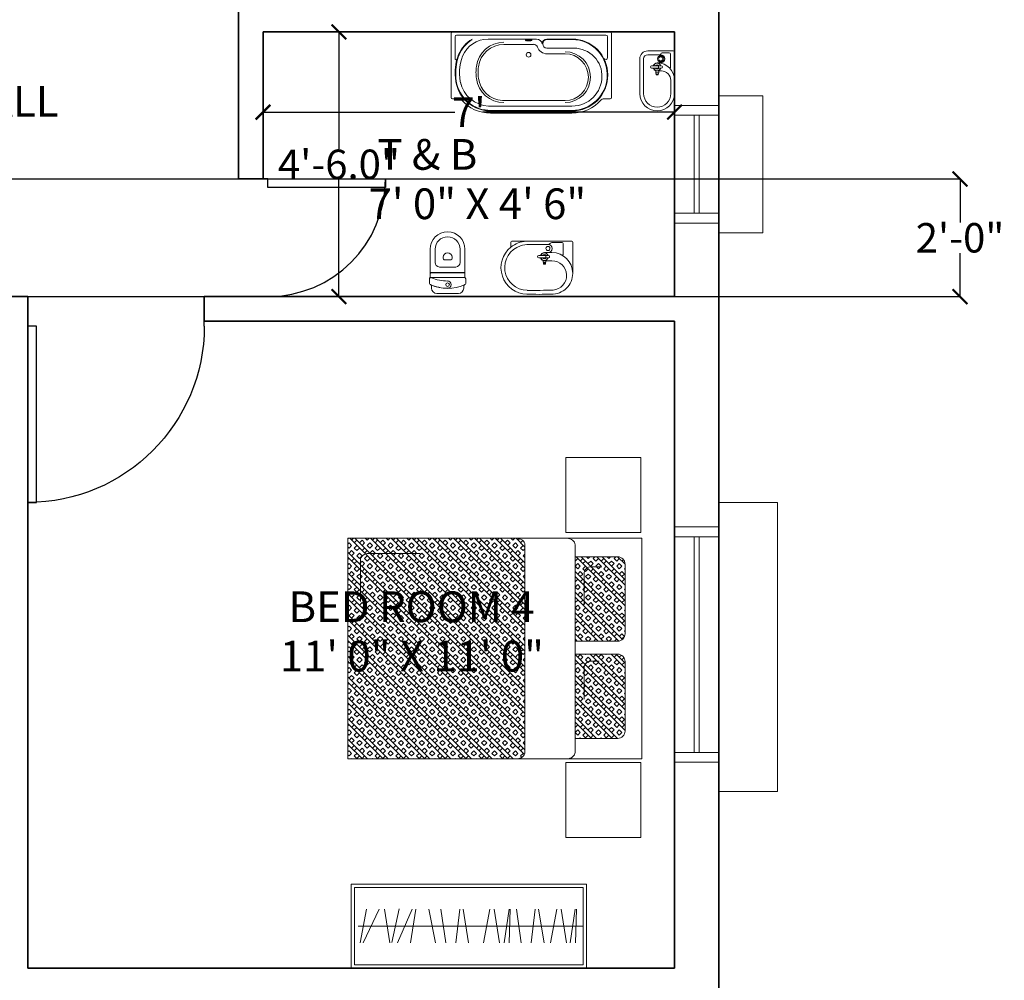
# Model space of a CAD drawing. Units: inches. Extents: x 844 to 2234, y 346 to 1084.
# Tile 43 of 93: x 1287 to 1488, y 627 to 823. Entities that reach past the tile are written whole.
import ezdxf

# ---------------------------------------------------------------- set-up
doc = ezdxf.new("R2010")
doc.units = ezdxf.units.IN
doc.header["$MEASUREMENT"] = 0
for name, color, linetype, lineweight in [('A-ANNO-DIMS', 2, 'Continuous', 18), ('A-AREA-IDEN', 7, 'Continuous', 18), ('A-FLOR-FIXT', 8, 'Continuous', 18), ('A-WALL', 7, 'Continuous', 35), ('beds', 130, 'Continuous', 18), ('doors', 170, 'Continuous', 25), ('furniture', 8, 'Continuous', 18), ('windows', 1, 'Continuous', 18)]:
    doc.layers.add(name, color=color, linetype=linetype, lineweight=lineweight)
doc.styles.get("Standard").update_dxf_attribs({"font": 'arial.ttf'})
doc.dimstyles.get("Standard").update_dxf_attribs({"dimtxt": 6, "dimasz": 3, "dimexe": 0.18, "dimexo": 0.0625, "dimgap": 0.09, "dimtad": 0, "dimtih": 1, "dimtoh": 1, "dimdec": 1, "dimzin": 0, "dimdsep": 46, "dimlunit": 3, "dimtxsty": 'Standard', "dimblk": 'ARCHTICK', "dimcen": 0.09, "dimadec": 0, "dimazin": 0, "dimtfac": 1, "dimtdec": 1, "dimtofl": 0, "dimtmove": 0, "dimatfit": 3, "dimfxl": 1, "dimtolj": 1, "dimtzin": 0, "dimarcsym": 0})
pattern_1 = [(135, (-1377.70473, -125.71507), (-0.070710678, -0.070710678), []), (135, (-1377.68705, -125.69739), (-0.070710678, -0.070710678), []), (45, (-1377.70473, -125.71507), (-0.070710678, 0.070710678), [-0.025, 0.025]), (45, (-1377.72241, -125.69739), (-0.070710678, 0.070710678), [-0.025, 0.025]), (45, (-1377.74009, -125.67972), (-0.070710678, 0.070710678), [0.025, -0.025]), (45, (-1377.75776, -125.66204), (-0.070710678, 0.070710678), [0.025, -0.025]), (135, (-1377.66938, -125.67972), (-0.070710678, -0.070710678), [0.025, -0.025]), (135, (-1377.6517, -125.66204), (-0.070710678, -0.070710678), [0.025, -0.025])]

# ---------------------------------------------------------------- blocks, each defined once
blk = doc.blocks.new('*U2')
for p, q in [((0, 0), (0, -6)), ((36, 0), (36, -6))]:
    blk.add_line(p, q)
blk.add_lwpolyline([(0, 0), (0, 36), (1.75, 36), (1.75, 0)], close=True)
blk.add_arc((0, 0), 36, 0, 90)
blk = doc.blocks.new('*U4')
for p, q in [((0, 0), (0, -6)), ((24, 0), (24, -6))]:
    blk.add_line(p, q)
blk.add_lwpolyline([(0, 0), (0, 24), (1.75, 24), (1.75, 0)], close=True)
blk.add_arc((0, 0), 24, 0, 90)
blk = doc.blocks.new('MAT-P10')
h = blk.add_hatch()
h.set_pattern_fill('BOX', color=256, scale=0.1, angle=45, style=0)
h.set_pattern_definition(pattern_1)
h.paths.add_polyline_path([(-0.1565, 1.4605), (0.417, 1.4605), (0.417, 1.7513, 0.414214), (0.367, 1.8013), (-0.1065, 1.8013, 0.414214), (-0.1565, 1.7513)])
h.paths.add_polyline_path([(0.5052, 1.4604), (1.0792, 1.4604), (1.0792, 1.7513, 0.414214), (1.0292, 1.8013), (0.5552, 1.8013, 0.414214), (0.5052, 1.7513)])
h = blk.add_hatch()
h.set_pattern_fill('BOX', color=256, scale=0.1, angle=45, style=0)
h.set_pattern_definition(pattern_1)
edge = h.paths.add_edge_path()
edge.add_line((1.2049, -0.085), (1.2049, 1.0625))
edge.add_ellipse((1.1608, 1.0627), major_axis=(0, 0.0568), ratio=0.776379, start_angle=270, end_angle=360)
edge.add_line((1.1608, 1.1195), (-0.251, 1.1195))
edge.add_ellipse((-0.251, 1.0627), major_axis=(0, 0.0568), ratio=0.776379, start_angle=0, end_angle=88.13958)
edge.add_line((-0.2951, 1.0641), (-0.2951, -0.085))
edge.add_line((-0.2951, -0.085), (1.2049, -0.085))
for p, q in [((-0.251, 1.4605), (1.1608, 1.4604)), ((-0.251, 1.1195), (1.1608, 1.1195)), ((1.1017, 0.406), (1.1017, 0.0572)), ((1.0576, 0.0004), (0.7754, 0.0004))]:
    blk.add_line(p, q)
for points in [[(-0.8301, 1.9091), (-0.3191, 1.9091), (-0.3191, 1.3981), (-0.8301, 1.3981)], [(1.2049, -0.085), (-0.2951, -0.085), (-0.2951, 1.9151), (1.2049, 1.915)], [(1.2441, 1.9091), (1.755, 1.9091), (1.755, 1.3981), (1.2441, 1.3981)]]:
    blk.add_lwpolyline(points, close=True)
for points in [[(0.417, 1.4604), (0.417, 1.7513, 0.414214), (0.367, 1.8013), (-0.1065, 1.8013, 0.414214), (-0.1565, 1.7513), (-0.1565, 1.4604)], [(1.0792, 1.4603), (1.0792, 1.7513, 0.414214), (1.0292, 1.8013), (0.5552, 1.8013, 0.414214), (0.5052, 1.7513), (0.5052, 1.4604)], [(0.3702, 1.6242), (0.3702, 1.5715, -0.414214), (0.3202, 1.5215), (0.1113, 1.5215)], [(1.0117, 1.6438), (1.0117, 1.5715, -0.414214), (0.9617, 1.5215), (0.7528, 1.5215)]]:
    blk.add_lwpolyline(points, format="xyb")
at = {"extrusion": (0, 0, -1)}
for centre, start_param, end_param in [((-0.251, 1.4036), 4.712389, 6.283185), ((1.1608, 1.4036), 0, 1.570796), ((-0.251, 1.0627), 4.712389, 6.283185), ((1.1608, 1.0627), 0, 1.570796), ((1.0576, 0.0572), 1.570796, 3.141593), ((1.0576, 0.0572), 1.570796, 3.141593)]:
    blk.add_ellipse(centre, major_axis=(0, 0.0568), ratio=0.776379, start_param=start_param, end_param=end_param, dxfattribs=at)
blk = doc.blocks.new('A$C7A17768A')
for p, q in [((-2.8, 0), (0, 0)), ((-2.8, -1), (-2.8, 0)), ((0, -1), (0, 0)), ((-2.76, -0.04), (-0.04, -0.04)), ((-2.76, -0.96), (-2.76, -0.04)), ((-0.04, -0.96), (-0.04, -0.04)), ((-2.617, -0.3), (-2.694, -0.7)), ((-2.66, -0.7), (-2.466, -0.3)), ((-2.403, -0.3), (-2.342, -0.7)), ((-2.229, -0.296), (-2.317, -0.696)), ((-2.074, -0.3), (-2.25, -0.7)), ((-2.096, -0.7), (-2.033, -0.3)), ((-1.875, -0.3), (-1.796, -0.7)), ((-1.732, -0.3), (-1.675, -0.7)), ((-1.555, -0.7), (-1.507, -0.3)), ((-1.467, -0.3), (-1.403, -0.7)), ((-1.227, -0.7), (-1.151, -0.3)), ((-1.098, -0.3), (-1.034, -0.7)), ((-0.98, -0.7), (-0.921, -0.3)), ((-0.908, -0.3), (-0.919, -0.7)), ((-0.834, -0.3), (-0.777, -0.7)), ((-0.657, -0.7), (-0.61, -0.3)), ((-0.57, -0.3), (-0.505, -0.7)), ((-0.429, -0.7), (-0.353, -0.3)), ((-0.301, -0.3), (-0.237, -0.7)), ((-0.192, -0.7), (-0.133, -0.3)), ((-0.12, -0.3), (-0.131, -0.7)), ((-0.04, -0.5), (-2.716, -0.5)), ((-2.8, -1), (0, -1)), ((-2.76, -0.96), (-0.04, -0.96))]:
    blk.add_line(p, q)
blk = doc.blocks.new('2SABICO')
at = {"color": 0, "linetype": 'ByBlock'}
for p, q in [((0.478, 0.195), (0.089, 0.195)), ((0.478, 0.152), (0.089, 0.152)), ((0, 0.106), (0, 0)), ((0, 0), (0, -0.18)), ((0.043, -0.039), (0.043, 0.106)), ((0.135, 0), (0.135, -0.003)), ((0.168, 0.064), (0.168, -0.015)), ((0.192, 0.064), (0.192, -0.015)), ((0.221, 0.012), (0.222, 0.012)), ((0.223, 0.016), (0.223, -0.016)), ((0.224, 0.017), (0.245, 0.017)), ((0.246, 0.016), (0.246, -0.016)), ((0.25, 0.014), (0.246, 0.014)), ((0.26, 0.01), (0.268, 0.01)), ((0.268, -0.01), (0.268, 0.01)), ((0.268, 0.01), (0.269, 0.009)), ((0.269, -0.009), (0.269, 0.009)), ((0.023, -0.057), (0.023, -0.135)), ((0.135, 0), (0.135, -0.039)), ((0.168, -0.015), (0.192, -0.015)), ((0.168, -0.015), (0.168, -0.046)), ((0.192, -0.015), (0.192, -0.046)), ((0.221, -0.012), (0.222, -0.012)), ((0.224, -0.017), (0.245, -0.017)), ((0.225, -0.017), (0.225, -0.047)), ((0.25, -0.014), (0.246, -0.014)), ((0.26, -0.01), (0.268, -0.01)), ((0.268, -0.01), (0.269, -0.009)), ((0.015, -0.195), (0.478, -0.195)), ((0.038, -0.15), (0.179, -0.15)), ((0.33, -0.152), (0.478, -0.152))]:
    blk.add_line(p, q, dxfattribs=at)
for radius in [0.035, 0.023]:
    blk.add_circle((0.089, -0.039), radius, dxfattribs=at)
for centre, radius, start, end in [((0.089, 0.106), 0.089, 90, 180), ((0.089, 0.106), 0.046, 90, 180), ((0.478, 0), 0.195, 270, 90), ((0.478, 0), 0.152, 270, 90), ((0.18, 0), 0.045, 105.6643, 180), ((0.18, 0), 0.042, 106.8152, 252.6853), ((0.18, 0), 0.0235, 121.1327, 237.8651), ((0.18, 0.064), 0.0121, 0, 180), ((0.18, 0), 0.045, 17.0576, 74.3357), ((0.18, 0), 0.042, 287.3147, 73.1848), ((0.18, 0), 0.0235, 302.1349, 58.8673), ((0.221, 0.013), 0.001, 197.9471, 270), ((0.222, 0.013), 0.001, 270, 0), ((0.224, 0.016), 0.001, 90, 180), ((0.245, 0.016), 0.001, 0, 90), ((0.25, 0), 0.0143, 270, 90), ((0.041, -0.057), 0.018, 99.5941, 180), ((0.037, -0.033), 0.006, 279.5941, 0), ((0.089, -0.039), 0.046, 180, 360), ((0.326, -0.003), 0.191, 180, 270), ((0.18, -0.046), 0.0125, 180, 0), ((0.221, -0.013), 0.001, 90, 162.0529), ((0.222, -0.013), 0.001, 0, 90), ((0.224, -0.016), 0.001, 180, 270), ((0.33, -0.047), 0.105, 180, 270), ((0.245, -0.016), 0.001, 270, 0), ((0.015, -0.18), 0.015, 180, 270), ((0.038, -0.135), 0.015, 180, 270), ((0.179, -0.14), 0.01, 270, 42.9682)]:
    blk.add_arc(centre, radius, start, end, dxfattribs=at)
blk = doc.blocks.new('2SAINCO')
at = {"color": 0, "linetype": 'ByBlock'}
for p, q in [((0, -0.121), (0, 0.121)), ((0.06, 0.181), (0.085, 0.181)), ((0.114, 0.203), (0.165, 0.203)), ((0.496, 0.195), (0.178, 0.195)), ((0.18, -0.188), (0.18, 0.188)), ((0.231, 0.185), (0.231, -0.185)), ((0.234, 0.185), (0.234, -0.185)), ((0.496, 0.14), (0.347, 0.14)), ((0.394, 0.05), (0.407, 0.05)), ((0.394, -0.05), (0.407, -0.05)), ((0.06, -0.181), (0.085, -0.181)), ((0.114, -0.201), (0.165, -0.201)), ((0.114, -0.203), (0.165, -0.203)), ((0.496, -0.195), (0.178, -0.195)), ((0.496, -0.14), (0.347, -0.14))]:
    blk.add_line(p, q, dxfattribs=at)
blk.add_circle((0.1, 0), 0.02, dxfattribs=at)
for centre, radius, start, end in [((0.06, 0.121), 0.06, 90, 180), ((0.517, 0), 0.46, 155.909, 204.091), ((0.085, 0.196), 0.015, 270, 344.534), ((0.114, 0.188), 0.015, 90, 164.534), ((0.165, 0.188), 0.015, 0, 90), ((0.221, 0.185), 0.01, 0, 90), ((0.224, 0.185), 0.01, 0, 90), ((0.347, 0.09), 0.05, 90, 177.3546), ((0.496, 0), 0.195, 270, 90), ((0.496, 0), 0.14, 270, 90), ((0.1, 0), 0.0405, 360, 180), ((0.517, 0), 0.458, 180, 204.67), ((0.66, 0.008), 0.52, 180.891, 201.3823), ((2.295, 0), 2, 177.3546, 182.6454), ((0.677, 0), 0.3, 172.9459, 187.0541), ((0.394, 0.035), 0.015, 90, 172.9459), ((0.407, 0), 0.05, 270, 90), ((0.347, -0.09), 0.05, 182.6454, 270), ((0.394, -0.035), 0.015, 187.0541, 270), ((0.06, -0.121), 0.06, 180, 270), ((0.085, -0.196), 0.015, 15.466, 90), ((0.114, -0.188), 0.015, 195.466, 270), ((0.114, -0.188), 0.013, 195.466, 270), ((0.165, -0.188), 0.013, 270, 30), ((0.165, -0.188), 0.015, 270, 0), ((0.221, -0.185), 0.01, 270, 0), ((0.224, -0.185), 0.01, 270, 0)]:
    blk.add_arc(centre, radius, start, end, dxfattribs=at)
blk = doc.blocks.new('2SABACO')
at = {"color": 0}
for p, q in [((1.341, 0.91), (0.429, 0.91)), ((1.341, 0.885), (0.429, 0.885)), ((1.341, 0.831), (0.407, 0.831)), ((1.341, 0.879), (0.429, 0.879)), ((-0.015, 0.735), (-0.015, 0.015)), ((0, 0.75), (0.08, 0.75)), ((1.263, 0.769), (0.562, 0.769)), ((1.77, 0.75), (1.69, 0.75)), ((1.785, 0.015), (1.785, 0.735)), ((0.03, 0.302), (0.03, 0.053)), ((1.263, 0.245), (1.06, 0.245)), ((1.74, 0.053), (1.74, 0.286)), ((0.578, 0.139), (0.911, 0.139)), ((1.363, 0.181), (1.06, 0.181)), ((0, 0), (1.77, 0)), ((0.048, 0.035), (1.722, 0.035)), ((0.401, 0.08), (0.942, 0.08)), ((1.343, 0.086), (1.06, 0.086)), ((1.343, 0.079), (1.06, 0.079))]:
    blk.add_line(p, q, dxfattribs=at)
blk.add_circle((0.855, 0.256), 0.026, dxfattribs=at)
for centre, radius, start, end in [((0.429, 0.48), 0.43, 90, 139.2943), ((0.429, 0.48), 0.405, 90, 98.9726), ((1.341, 0.48), 0.43, 40.7057, 90), ((1.341, 0.485), 0.401, 359.4627, 90), ((0.428, 0.49), 0.395, 98.9726, 181.1954), ((0.428, 0.49), 0.389, 98.9726, 181.2301), ((0.425, 0.49), 0.342, 93.1008, 168.0202), ((0.578, 0.481), 0.311, 90, 172.609), ((0.429, 0.48), 0.399, 90, 98.9726), ((1.263, 0.507), 0.285, 270, 90), ((1.341, 0.485), 0.394, 3.5237, 90), ((1.341, 0.495), 0.336, 0, 90), ((0, 0.735), 0.015, 90, 180), ((0.08, 0.78), 0.03, 270, 319.2943), ((0.578, 0.481), 0.288, 93.3767, 172.609), ((1.263, 0.507), 0.262, 270, 90), ((1.69, 0.78), 0.03, 220.7057, 270), ((1.77, 0.735), 0.015, 0, 90), ((0.559, 0.454), 0.48, 163.1286, 202.3619), ((0.559, 0.454), 0.528, 177.0415, 202.3619), ((0.559, 0.454), 0.521, 177.0156, 202.3619), ((0.79, 0.454), 0.525, 172.609, 180), ((0.79, 0.454), 0.525, 180, 187.391), ((0.79, 0.454), 0.502, 172.609, 180), ((0.79, 0.454), 0.502, 180, 187.391), ((1.343, 0.477), 0.392, 270, 4.5675), ((1.343, 0.477), 0.398, 270, 0.539), ((1.363, 0.495), 0.314, 270, 2.2815), ((0.578, 0.427), 0.311, 187.391, 270), ((0.578, 0.427), 0.288, 187.391, 270), ((0.042, 0.302), 0.0116, 16.3184, 180.0001), ((0.401, 0.389), 0.357, 202.3619, 239.8287), ((0.401, 0.389), 0.351, 202.3619, 239.2093), ((0.401, 0.389), 0.309, 202.3619, 270), ((1.06, 0.133), 0.112, 90, 161.2369), ((1.718, 0.286), 0.0222, 0, 152.9966), ((0.911, 0.183), 0.045, 270, 341.2369), ((0.942, 0.145), 0.065, 270, 349.4977), ((1.06, 0.133), 0.054, 180, 270), ((1.06, 0.133), 0.0475, 90, 270), ((0, 0.015), 0.015, 180, 270), ((0.048, 0.053), 0.018, 180, 270), ((0.559, 0.454), 0.48, 250.7818, 251.0555), ((0.821, 0.092), 0.00282, 119.7759, 180), ((0.821, 0.092), 0.00282, 180, 240.2241), ((0.837, 0.064), 0.0347, 103.3326, 119.7759), ((0.835, 0.025), 0.071, 96.5949, 102.1924), ((0.837, 0.12), 0.0347, 240.2241, 256.6674), ((0.847, -0.08), 0.177, 92.7417, 96.5949), ((0.848, 0.02), 0.0808, 95.6065, 103.3326), ((0.848, 0.164), 0.0808, 256.6674, 264.3935), ((0.855, -0.252), 0.349, 90, 92.7417), ((0.855, -0.053), 0.153, 90, 95.6065), ((0.855, 0.237), 0.153, 264.3935, 270), ((0.855, -0.053), 0.153, 84.3935, 90), ((0.855, -0.252), 0.349, 87.2583, 90), ((0.855, 0.237), 0.153, 270, 275.6065), ((0.862, 0.02), 0.0808, 76.6674, 84.3935), ((0.862, 0.164), 0.0808, 275.6065, 283.3326), ((0.863, -0.08), 0.177, 83.4051, 87.2583), ((0.873, 0.064), 0.0347, 60.2241, 76.6674), ((0.873, 0.12), 0.0347, 283.3326, 299.7759), ((0.875, 0.025), 0.071, 77.8076, 83.4051), ((0.889, 0.092), 0.00282, 360, 60.2241), ((0.889, 0.092), 0.00282, 299.7759, 360), ((1.722, 0.053), 0.018, 270, 0), ((1.77, 0.015), 0.015, 270, 0)]:
    blk.add_arc(centre, radius, start, end, dxfattribs=at)
blk = doc.blocks.new('2SALACO2')
at = {"color": 0}
for p, q in [((0, 0), (-0.392, 0)), ((0.28, 0), (0, 0)), ((-0.402, -0.01), (-0.402, -0.36)), ((-0.293, -0.026), (-0.293, -0.15)), ((-0.283, -0.016), (-0.166, -0.016)), ((-0.112, -0.035), (-0.133, -0.035)), ((-0.124, -0.035), (0.09, -0.035)), ((0.29, -0.01), (0.29, -0.064)), ((-0.169, -0.128), (-0.085, -0.128)), ((-0.102, -0.219), (-0.169, -0.219)), ((-0.1, -0.161), (-0.131, -0.161)), ((-0.1, -0.186), (-0.131, -0.186)), ((-0.102, -0.217), (-0.102, -0.234)), ((-0.07, -0.216), (-0.101, -0.216)), ((-0.1, -0.161), (-0.1, -0.186)), ((-0.021, -0.161), (-0.1, -0.161)), ((-0.021, -0.186), (-0.1, -0.186)), ((-0.098, -0.214), (-0.098, -0.216)), ((-0.073, -0.214), (-0.073, -0.216)), ((-0.069, -0.217), (-0.069, -0.234)), ((-0.07, -0.235), (-0.101, -0.235)), ((-0.097, -0.239), (-0.098, -0.241)), ((-0.098, -0.241), (-0.098, -0.248)), ((-0.098, -0.241), (-0.073, -0.241)), ((-0.073, -0.248), (-0.098, -0.248)), ((-0.097, -0.235), (-0.097, -0.239)), ((-0.074, -0.239), (-0.097, -0.239)), ((-0.097, -0.248), (-0.097, -0.256)), ((-0.073, -0.256), (-0.097, -0.256)), ((-0.097, -0.256), (-0.094, -0.257)), ((-0.077, -0.257), (-0.094, -0.257)), ((-0.073, -0.256), (-0.077, -0.257)), ((-0.074, -0.235), (-0.074, -0.239)), ((-0.074, -0.239), (-0.073, -0.241)), ((-0.073, -0.241), (-0.073, -0.248)), ((-0.073, -0.248), (-0.073, -0.256))]:
    blk.add_line(p, q, dxfattribs=at)
blk.add_lwpolyline([(-0.402, -0.36, 0.423787), (-0.161, -0.593, 0.423787)], format="xyb", dxfattribs=at)
blk.add_circle((-0.124, -0.081), 0.023, dxfattribs=at)
for centre, radius, start, end in [((-0.392, -0.01), 0.01, 90, 180), ((0.28, -0.01), 0.01, 0, 90), ((-0.283, -0.026), 0.01, 90, 180), ((-0.124, -0.081), 0.0462, 90, 270), ((-0.166, -0.046), 0.03, 31.2573, 90), ((-0.133, -0.026), 0.009, 211.2573, 270), ((0.09, -0.29), 0.255, 68.9449, 90), ((0.105, -0.295), 0.255, 271.0077, 72.4499), ((0.105, -0.297), 0.297, 271.4871, 51.4524), ((0.105, -0.297), 0.297, 51.4524, 87.1707), ((-0.169, -0.36), 0.233, 90, 180), ((-0.169, -0.383), 0.164, 90, 265.4963), ((-0.285, -0.15), 0.008, 180, 299.1062), ((-0.131, -0.173), 0.0125, 90, 270), ((-0.085, -0.173), 0.042, 16.8152, 162.6853), ((-0.085, -0.173), 0.042, 197.3147, 343.1848), ((-0.085, -0.173), 0.0235, 31.1327, 147.8651), ((-0.085, -0.173), 0.0235, 212.1349, 328.8673), ((-0.101, -0.217), 0.001, 90, 180), ((-0.085, -0.173), 0.0458, 15.3964, 90), ((-0.085, -0.173), 0.0458, 289.9182, 344.6036), ((-0.07, -0.217), 0.001, 0, 90), ((-0.021, -0.173), 0.0121, 270, 90), ((-0.101, -0.234), 0.001, 180, 270), ((-0.07, -0.234), 0.001, 270, 0), ((0.021, 4.449), 5, 267.6742, 271.0081), ((-0.017, 4.405), 5, 268.3511, 271.4874)]:
    blk.add_arc(centre, radius, start, end, dxfattribs=at)
blk = doc.blocks.new('_ArchTick')
at = {"color": 0, "linetype": 'ByBlock', "const_width": 0.15}
blk.add_lwpolyline([(-0.5, -0.5), (0.5, 0.5)], dxfattribs=at)
blk = doc.blocks.new('*D41')
at = {"layer": 'A-ANNO-DIMS', "color": 0, "lineweight": -2, "transparency": 16777216}
for p, q in [((1362.73, 820.31), (1351.92, 820.31)), ((1352.1, 820.31), (1352.1, 796.46)), ((1352.1, 766.31), (1352.1, 790.16)), ((1362.73, 766.31), (1351.92, 766.31))]:
    blk.add_line(p, q, dxfattribs=at)
at = {"layer": 'Defpoints', "color": 0, "transparency": 16777216}
for p in [(1362.79, 820.31), (1352.1, 766.31), (1362.79, 766.31)]:
    blk.add_point(p, dxfattribs=at)
at = {"layer": 'A-ANNO-DIMS', "color": 0, "lineweight": -2, "transparency": 16777216, "xscale": 3, "yscale": 3, "zscale": 3}
for p, rotation in [((1352.1, 820.31), 90), ((1352.1, 766.31), 270)]:
    blk.add_blockref('_ArchTick', p, dxfattribs=dict(at, rotation=rotation))
at = {"layer": 'A-ANNO-DIMS', "color": 0, "transparency": 16777216, "insert": (1352.1, 793.31), "char_height": 6, "attachment_point": 5}
blk.add_mtext('\\A1;4\'-6.0"', dxfattribs=at)
blk = doc.blocks.new('*D42')
at = {"layer": 'A-ANNO-DIMS', "color": 0, "lineweight": -2, "transparency": 16777216}
for p, q in [((1336.62, 804.01), (1336.62, 804.13)), ((1336.62, 803.95), (1375.79, 803.95)), ((1420.62, 803.95), (1381.44, 803.95)), ((1420.62, 804.01), (1420.62, 804.13))]:
    blk.add_line(p, q, dxfattribs=at)
at = {"layer": 'Defpoints', "color": 0, "transparency": 16777216}
for p in [(1336.62, 803.95), (1336.62, 803.95), (1420.62, 803.95)]:
    blk.add_point(p, dxfattribs=at)
at = {"layer": 'A-ANNO-DIMS', "color": 0, "lineweight": -2, "transparency": 16777216, "xscale": 3, "yscale": 3, "zscale": 3, "rotation": 180}
blk.add_blockref('_ArchTick', (1336.62, 803.95), dxfattribs=at)
at = {"layer": 'A-ANNO-DIMS', "color": 0, "lineweight": -2, "transparency": 16777216, "xscale": 3, "yscale": 3, "zscale": 3}
blk.add_blockref('_ArchTick', (1420.62, 803.95), dxfattribs=at)
at = {"layer": 'A-ANNO-DIMS', "color": 0, "transparency": 16777216, "insert": (1378.62, 803.95), "char_height": 6, "attachment_point": 5}
blk.add_mtext("\\A1;7'", dxfattribs=at)
blk = doc.blocks.new('WIN-48IN')
for p, q in [((0, 9), (0, 21)), ((0, 21), (59, 21)), ((59, 9), (59, 21)), ((6, 9), (0, 9)), ((54, 9), (6, 9)), ((6, 9), (6, 0)), ((8, 9), (8, 0)), ((52, 0), (52, 9)), ((54, 0), (54, 9)), ((54, 9), (59, 9)), ((8, 5), (52, 5)), ((8, 4), (52, 4)), ((6, 0), (54, 0))]:
    blk.add_line(p, q)
blk = doc.blocks.new('WIN-24IN')
for p, q in [((9, 28), (0, 28)), ((0, 0), (0, 28)), ((9, 26), (9, 28)), ((18, 26), (9, 26)), ((9, 26), (9, 2)), ((18, 2), (18, 26)), ((18, 24), (9, 24)), ((13, 4), (13, 24)), ((14, 4), (14, 24)), ((9, 4), (18, 4)), ((9, 2), (18, 2)), ((9, 2), (9, 0)), ((9, 0), (0, 0))]:
    blk.add_line(p, q)
blk = doc.blocks.new('*D111')
at = {"layer": 'A-ANNO-DIMS', "color": 0, "lineweight": -2, "transparency": 16777216}
for p, q in [((1420.68, 842.06), (1422.66, 842.06)), ((1422.48, 842.06), (1422.48, 839.04)), ((1422.48, 829.64), (1422.48, 832.66)), ((1420.68, 829.64), (1422.66, 829.64))]:
    blk.add_line(p, q, dxfattribs=at)
at = {"layer": 'Defpoints', "color": 0, "transparency": 16777216}
for p in [(1420.62, 842.06), (1422.48, 842.06), (1420.62, 829.64)]:
    blk.add_point(p, dxfattribs=at)
at = {"layer": 'A-ANNO-DIMS', "color": 0, "lineweight": -2, "transparency": 16777216, "xscale": 3, "yscale": 3, "zscale": 3}
for p, rotation in [((1422.48, 842.06), 90), ((1422.48, 829.64), 270)]:
    blk.add_blockref('_ArchTick', p, dxfattribs=dict(at, rotation=rotation))
at = {"layer": 'A-ANNO-DIMS', "color": 0, "transparency": 16777216, "insert": (1422.48, 835.85), "char_height": 6, "attachment_point": 5}
blk.add_mtext('\\A1;BIDET 1\'-0 1/2" TYP.', dxfattribs=at)
blk = doc.blocks.new('*D149')
at = {"layer": 'A-ANNO-DIMS', "color": 0, "lineweight": -2, "transparency": 16777216}
for p, q in [((1043.68, 790.31), (1479.05, 790.31)), ((1478.87, 790.31), (1478.87, 781.46)), ((1478.87, 766.31), (1478.87, 775.16)), ((1043.68, 766.31), (1479.05, 766.31))]:
    blk.add_line(p, q, dxfattribs=at)
at = {"layer": 'Defpoints', "color": 0, "transparency": 16777216}
for p in [(1043.62, 790.31), (1478.87, 790.31), (1043.62, 766.31)]:
    blk.add_point(p, dxfattribs=at)
at = {"layer": 'A-ANNO-DIMS', "color": 0, "lineweight": -2, "transparency": 16777216, "xscale": 3, "yscale": 3, "zscale": 3}
for p, rotation in [((1478.87, 790.31), 90), ((1478.87, 766.31), 270)]:
    blk.add_blockref('_ArchTick', p, dxfattribs=dict(at, rotation=rotation))
at = {"layer": 'A-ANNO-DIMS', "color": 0, "transparency": 16777216, "insert": (1478.87, 778.31), "char_height": 6, "attachment_point": 5}
blk.add_mtext('\\A1;2\'-0"', dxfattribs=at)

msp = doc.modelspace()

# ---------------------------------------------------------------- linework, layer by layer
at = {"layer": 'A-WALL'}
for p, q in [((1429.62, 1025.31), (1429.62, 430.31)), ((1331.62, 879.31), (1331.62, 790.31)), ((1420.62, 820.31), (1336.62, 820.31)), ((1336.62, 820.31), (1336.62, 790.31)), ((1420.62, 820.31), (1420.62, 766.31)), ((1331.62, 790.31), (1336.62, 790.31)), ((1288.62, 766.31), (1283.62, 766.31)), ((1288.62, 761.31), (1288.62, 766.31)), ((1331.62, 766.31), (1324.62, 766.31)), ((1324.62, 761.31), (1324.62, 766.31)), ((1331.62, 766.31), (1336.62, 766.31)), ((1420.62, 766.31), (1336.62, 766.31)), ((1288.62, 761.31), (1288.62, 629.31)), ((1420.62, 761.31), (1324.62, 761.31)), ((1420.62, 761.31), (1420.62, 629.31)), ((1420.62, 629.31), (1288.62, 629.31))]:
    msp.add_line(p, q, dxfattribs=at)

# ---------------------------------------------------------------- block references
at = {"layer": 'A-FLOR-FIXT', "xscale": -18.21101258924898, "yscale": 18.21101258924898, "zscale": 18.21101258924898}
for name, p, rotation in [('2SABACO', (1375.25, 820.31), 180), ('2SABICO', (1417.06, 816.45), 90), ('2SAINCO', (1374.28, 766.94), 270)]:
    msp.add_blockref(name, p, dxfattribs=dict(at, rotation=rotation))
msp.add_blockref('2SALACO2', (1392.5, 777.61), dxfattribs=at)
at = {"layer": 'beds', "xscale": -29.99962925113936, "yscale": 29.99962925113936, "zscale": 29.99962925113936, "rotation": 270}
msp.add_blockref('MAT-P10', (1356.48, 680.85), dxfattribs=at)
at = {"layer": 'doors', "rotation": 270}
msp.add_blockref('*U4', (1337.62, 790.31), dxfattribs=at)
at = {"layer": 'doors', "xscale": -1, "rotation": 180}
msp.add_blockref('*U2', (1288.62, 760.31), dxfattribs=at)
at = {"layer": 'furniture', "xscale": 17.14285714285603, "yscale": 17.14285714285603, "zscale": 17.14285714285603}
msp.add_blockref('A$C7A17768A', (1402.62, 646.45), dxfattribs=at)
at = {"layer": 'windows', "rotation": 180}
msp.add_blockref('WIN-24IN', (1438.62, 807.31), dxfattribs=at)
at = {"layer": 'windows', "extrusion": (0, 0, -1), "zscale": -1, "rotation": 90.00000000000178}
msp.add_blockref('WIN-48IN', (-1420.62, 665.31), dxfattribs=at)

# ---------------------------------------------------------------- texts
at = {"layer": 'A-AREA-IDEN'}
for s, height, p in [('DINING HALL', 6.2688, (1243.09, 803)), ('T & B', 6.269, (1359.95, 792.19)), (' 7\' 0" X 4\' 6"', 6.2688, (1356.25, 782.12)), ('BED ROOM 4', 6.269, (1341.83, 699.89)), (' 11\' 0" X 11\' 0"', 6.2688, (1338.13, 689.82))]:
    msp.add_text(s, height=height, dxfattribs=at).set_placement(p)

# ---------------------------------------------------------------- dimensions: what is measured, and where the dimension line sits
at = {"layer": 'A-ANNO-DIMS'}
dim = msp.add_linear_dim(base=(1422.48, 842.06), p1=(1420.62, 829.64), p2=(1420.62, 842.06), angle=90, text='BIDET <> TYP.', dimstyle='Standard', override={"dimdec": 1, "dimlfac": 1, "dimrnd": 0, "dimzin": 1, "dimdsep": 46, "dimlunit": 4, "dimfrac": 2}, dxfattribs=at)
dim.commit()
dim.dimension.update_dxf_attribs({"geometry": '*D111', "text_midpoint": (1422.48, 835.85)})
for base, p1, p2, override, picture, middle in [((1352.1, 766.31), (1362.79, 820.31), (1362.79, 766.31), {"dimclrd": 0, "dimclre": 0, "dimclrt": 0}, '*D41', (1352.1, 793.31)), ((1478.87, 790.31), (1043.62, 766.31), (1043.62, 790.31), {"dimdec": 1, "dimlfac": 1, "dimrnd": 0, "dimzin": 1, "dimdsep": 46, "dimlunit": 4, "dimfrac": 2}, '*D149', (1478.87, 778.31))]:
    dim = msp.add_linear_dim(base=base, p1=p1, p2=p2, angle=90, dimstyle='Standard', override=override, dxfattribs=at)
    dim.commit()
    dim.dimension.update_dxf_attribs({"geometry": picture, "text_midpoint": middle})
dim = msp.add_linear_dim(base=(1336.62, 803.95), p1=(1420.62, 803.95), p2=(1336.62, 803.95), dimstyle='Standard', override={"dimclrd": 0, "dimclre": 0, "dimclrt": 0}, dxfattribs=at)
dim.commit()
dim.dimension.update_dxf_attribs({"geometry": '*D42', "text_midpoint": (1378.62, 803.95)})

doc.saveas('drawing.dxf')
